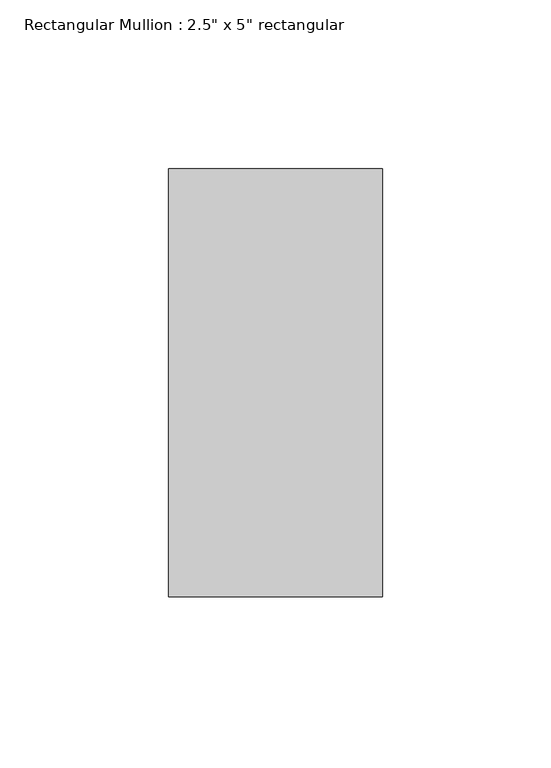
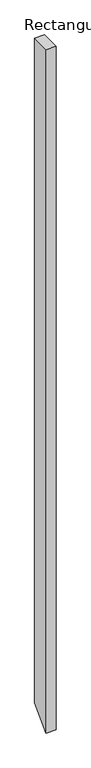
"""IFC4 building model written with IfcOpenShell, lengths in millimetres: member geometry."""

from ifc_helpers import new_model, si_unit, frame, origin, place, context, project, spatial, polyline, outline, extrude, source, transform, mapped, element, save


def member_f377c62d(model_context):
    return source(origin(), model_context, "Body", "SweptSolid", [
        extrude(outline(polyline([(-63.5, 0.0), (63.5, 0.0), (63.5, -4491.532599), (-63.5, -4618.532599), (-63.5, 0.0)])), frame((-63.5, 0.0, 0.0), z_axis=(1.0, 0.0, 0.0), x_axis=(0.0, 1.0, 0.0)), (0.0, 0.0, 1.0), 63.5),
    ])


if __name__ == "__main__":
    model = new_model("IFC4")
    model_context = context("Model", 3, world=origin())
    ifc_project = project(units=[si_unit("LENGTHUNIT", "METRE", prefix="MILLI")], contexts=[model_context])
    site = spatial("IfcSite", under=ifc_project)
    building = spatial("IfcBuilding", under=site)
    placement = place(None, origin())
    member_shape = member_f377c62d(model_context)
    element("IfcMember", 1, ObjectType="Rectangular Mullion : 2.5\" x 5\" rectangular", at=placement, inside=building, context=model_context, shape_type="MappedRepresentation", body=[
        mapped(member_shape, transform((0.0, 0.0, 0.0), x_axis=(1.0, 0.0, 0.0), y_axis=(0.0, 1.0, 0.0), z_axis=(0.0, 0.0, 1.0))),
    ])
    save(model, "model.ifc")

# Revit data of these elements
# Type "Rectangular Mullion : 2.5\" x 5\" rectangular"
#   built-in parameter 1007304 = 0.416667 (stored number, unit not read)
#   built-in parameter 1007301 = 0.104167 (stored number, unit not read)
#   built-in parameter 1007300 = 0.104167 (stored number, unit not read)
# Element 1 (IfcMember, "Rectangular Mullion : 2.5\" x 5\" rectangular")
#   Materials on its faces: "Aluminum"
# Materials
#   "Aluminum": class "Metal", colour RGB 247 247 247, transparency 0, Description = "Aluminum 6061", Cost = 0
